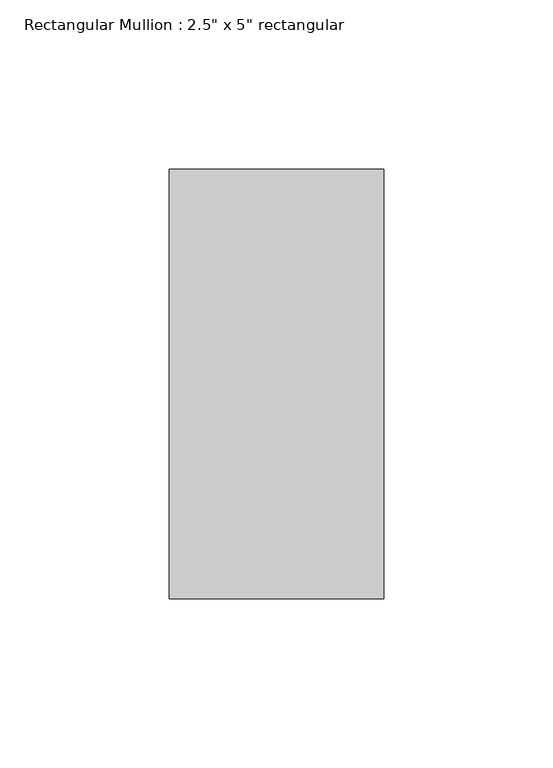
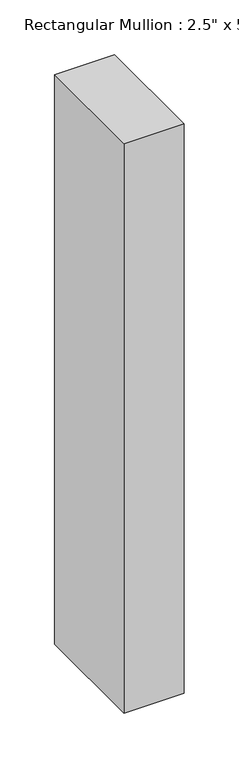
"""IFC4 building model written with IfcOpenShell, lengths in millimetres: member geometry."""

from ifc_helpers import new_model, si_unit, frame, origin, place, context, project, spatial, polyline, outline, extrude, source, transform, mapped, element, save


def member_12300432(model_context):
    return source(origin(), model_context, "Body", "SweptSolid", [
        extrude(outline(polyline([(31.75, 63.5), (31.75, -63.5), (-31.75, -63.5), (-31.75, 63.5), (31.75, 63.5)])), frame((0.0, 0.0, -635.0), z_axis=(0.0, 0.0, 1.0), x_axis=(1.0, 0.0, 0.0)), (0.0, 0.0, 1.0), 635.0),
    ])


if __name__ == "__main__":
    model = new_model("IFC4")
    model_context = context("Model", 3, world=origin())
    ifc_project = project(units=[si_unit("LENGTHUNIT", "METRE", prefix="MILLI")], contexts=[model_context])
    site = spatial("IfcSite", under=ifc_project)
    building = spatial("IfcBuilding", under=site)
    placement = place(None, origin())
    member_shape = member_12300432(model_context)
    element("IfcMember", 1, ObjectType="Rectangular Mullion : 2.5\" x 5\" rectangular", at=placement, inside=building, context=model_context, shape_type="MappedRepresentation", body=[
        mapped(member_shape, transform((0.0, 0.0, 0.0), x_axis=(1.0, 0.0, 0.0), y_axis=(0.0, 1.0, 0.0), z_axis=(0.0, 0.0, 1.0))),
    ])
    save(model, "model.ifc")

# Revit data of these elements
# Type "Rectangular Mullion : 2.5\" x 5\" rectangular"
#   built-in parameter 1007304 = 0.416667 (stored number, unit not read)
#   built-in parameter 1007301 = 0.104167 (stored number, unit not read)
#   built-in parameter 1007300 = 0.104167 (stored number, unit not read)
# Element 1 (IfcMember, "Rectangular Mullion : 2.5\" x 5\" rectangular")
#   Materials on its faces: "Aluminum"
# Materials
#   "Aluminum": class "Metal", colour RGB 247 247 247, transparency 0, Description = "Aluminum 6061", Cost = 0
